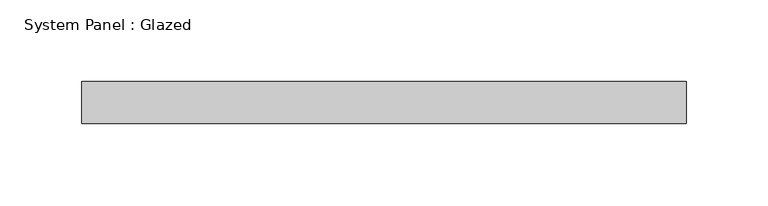
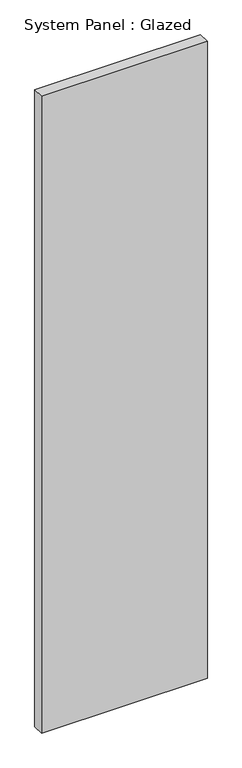
"""IFC4 building model written with IfcOpenShell, lengths in millimetres: plate geometry, System Panel : Glazed."""

from ifc_helpers import new_model, si_unit, origin, origin_with_axes, place, context, project, spatial, polyline, outline, extrude, source, transform, mapped, element, save


def system_panel_glazed_d172bbbe(model_context):
    return source(origin(), model_context, "Body", "SweptSolid", [
        extrude(outline(polyline([(184.15, 19.05), (-184.15, 19.05), (-184.15, 44.45), (184.15, 44.45), (184.15, 19.05)])), origin_with_axes(), (0.0, 0.0, 1.0), 1492.7840707),
    ])


if __name__ == "__main__":
    model = new_model("IFC4")
    model_context = context("Model", 3, world=origin())
    ifc_project = project(units=[si_unit("LENGTHUNIT", "METRE", prefix="MILLI")], contexts=[model_context])
    site = spatial("IfcSite", under=ifc_project)
    building = spatial("IfcBuilding", under=site)
    placement = place(None, origin())
    system_panel_glazed_shape = system_panel_glazed_d172bbbe(model_context)
    element("IfcPlate", 1, ObjectType="System Panel : Glazed", at=placement, inside=building, context=model_context, shape_type="MappedRepresentation", body=[
        mapped(system_panel_glazed_shape, transform((0.0, 0.0, 0.0), x_axis=(1.0, 0.0, 0.0), y_axis=(0.0, 1.0, 0.0), z_axis=(0.0, 0.0, 1.0))),
    ])
    save(model, "model.ifc")

# Revit data of these elements
# Type "System Panel : Glazed"
#   Construction Type Id = "GSP4R"
#   Analytic Construction = "1/8 in Pilkington single glazing"
#   Visual Light Transmittance = 0.9
#   Solar Heat Gain Coefficient = 0.86
#   Heat Transfer Coefficient (U) = 1.18115 BTU/(h·ft²·°F)
#   Define Thermal Properties by = 1
# Element 1 (IfcPlate, "System Panel : Glazed")
#   Materials on its faces: "Glass"
# Materials
#   "Glass": class "Glass", colour RGB 0 128 192, transparency 0.75, Description = "Soda Lime Glass", Cost = 0
